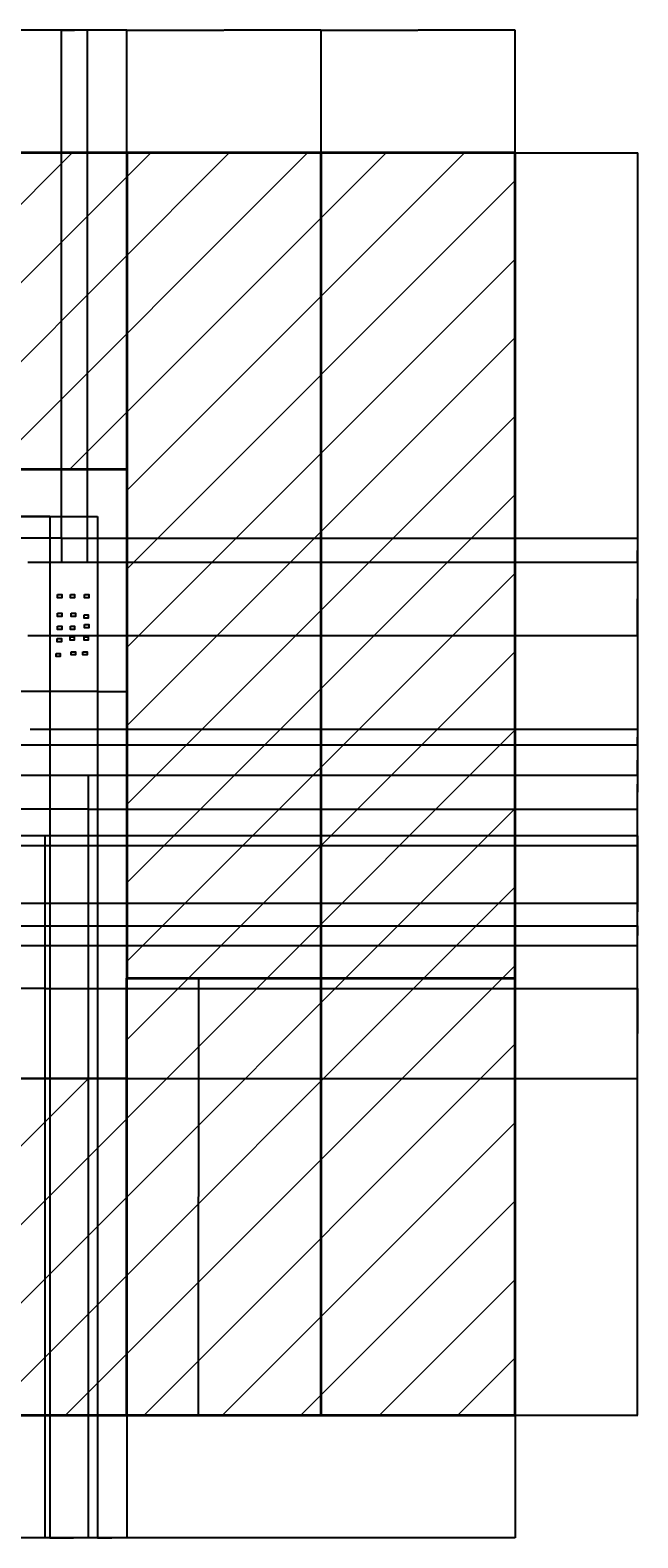
# Model space of a CAD drawing. Units: millimetres. Extents: x 2212 to 7718, y 1114 to 4219.
# Tile 5 of 5: x 6466 to 7718, y 1114 to 4219. Entities that reach past the tile are written whole.
import ezdxf

# ---------------------------------------------------------------- set-up
doc = ezdxf.new("R2010")
doc.units = ezdxf.units.MM
for name, color, linetype, lineweight in [('A-ANNO-DIMS', 2, 'Continuous', 18), ('A-ELEV-PATT', 8, 'Continuous', 13), ('A-EQPM', 4, 'Continuous', 25), ('A-FURN', 7, 'Continuous', 35)]:
    doc.layers.add(name, color=color, linetype=linetype, lineweight=lineweight)
doc.styles.get("Standard").update_dxf_attribs({"font": 'arial.ttf'})
doc.dimstyles.get("Standard").update_dxf_attribs({"dimtxt": 0.18, "dimasz": 0.18, "dimexe": 0.18, "dimexo": 0.0625, "dimgap": 0.09, "dimtad": 0, "dimtih": 1, "dimtoh": 1, "dimdec": 4, "dimzin": 0, "dimdsep": 46, "dimtxsty": 'Standard', "dimcen": 0.09, "dimadec": 0, "dimazin": 0, "dimtfac": 1, "dimtdec": 4, "dimtofl": 0, "dimtmove": 0, "dimatfit": 3, "dimfxl": 1, "dimtolj": 1, "dimtzin": 0, "dimarcsym": 0})

# ---------------------------------------------------------------- blocks, each defined once
blk = doc.blocks.new('*D7')
at = {"layer": 'A-ANNO-DIMS', "color": 0, "lineweight": -2, "transparency": 16777216}
for p, q in [((5865.1, 3966.2), (5865.1, 4218.9)), ((5865.3, 4218.7), (6264.9, 4218.7)), ((6665, 4218.7), (6265.4, 4218.7)), ((6665.1, 3966.2), (6665.1, 4218.9))]:
    blk.add_line(p, q, dxfattribs=at)
at = {"layer": 'A-ANNO-DIMS', "color": 0, "transparency": 16777216}
for points in [[(5865.3, 4218.7), (5865.3, 4218.7), (5865.1, 4218.7)], [(6665, 4218.7), (6665, 4218.7), (6665.1, 4218.7)]]:
    blk.add_solid(points, dxfattribs=at)
at = {"layer": 'Defpoints', "color": 0, "transparency": 16777216}
for p in [(6665.1, 4218.7), (5865.1, 3966.2), (6665.1, 3966.2)]:
    blk.add_point(p, dxfattribs=at)
at = {"layer": 'A-ANNO-DIMS', "color": 0, "transparency": 16777216, "insert": (6265.1, 4218.7), "char_height": 0.18, "attachment_point": 5}
blk.add_mtext('\\A1;800', dxfattribs=at)
blk = doc.blocks.new('*D8')
at = {"layer": 'A-ANNO-DIMS', "color": 0, "lineweight": -2, "transparency": 16777216}
for p, q in [((6665.1, 3966.2), (6665.1, 4218.9)), ((6665.3, 4218.7), (6864.8, 4218.7)), ((7065, 4218.7), (6865.4, 4218.7)), ((7065.1, 3966.2), (7065.1, 4218.9))]:
    blk.add_line(p, q, dxfattribs=at)
at = {"layer": 'A-ANNO-DIMS', "color": 0, "transparency": 16777216}
for points in [[(6665.3, 4218.7), (6665.3, 4218.7), (6665.1, 4218.7)], [(7065, 4218.7), (7065, 4218.7), (7065.1, 4218.7)]]:
    blk.add_solid(points, dxfattribs=at)
at = {"layer": 'Defpoints', "color": 0, "transparency": 16777216}
for p in [(7065.1, 4218.7), (6665.1, 3966.2), (7065.1, 3966.2)]:
    blk.add_point(p, dxfattribs=at)
at = {"layer": 'A-ANNO-DIMS', "color": 0, "transparency": 16777216, "insert": (6865.1, 4218.7), "char_height": 0.18, "attachment_point": 5}
blk.add_mtext('\\A1;400', dxfattribs=at)
blk = doc.blocks.new('*D9')
at = {"layer": 'A-ANNO-DIMS', "color": 0, "lineweight": -2, "transparency": 16777216}
for p, q in [((7065.1, 3966.2), (7065.1, 4218.9)), ((7065.3, 4218.7), (7264.8, 4218.7)), ((7465, 4218.7), (7265.4, 4218.7)), ((7465.1, 3966.2), (7465.1, 4218.9))]:
    blk.add_line(p, q, dxfattribs=at)
at = {"layer": 'A-ANNO-DIMS', "color": 0, "transparency": 16777216}
for points in [[(7065.3, 4218.7), (7065.3, 4218.7), (7065.1, 4218.7)], [(7465, 4218.7), (7465, 4218.7), (7465.1, 4218.7)]]:
    blk.add_solid(points, dxfattribs=at)
at = {"layer": 'Defpoints', "color": 0, "transparency": 16777216}
for p in [(7465.1, 4218.7), (7065.1, 3966.2), (7465.1, 3966.2)]:
    blk.add_point(p, dxfattribs=at)
at = {"layer": 'A-ANNO-DIMS', "color": 0, "transparency": 16777216, "insert": (7265.1, 4218.7), "char_height": 0.18, "attachment_point": 5}
blk.add_mtext('\\A1;400', dxfattribs=at)
blk = doc.blocks.new('*D18')
at = {"layer": 'A-ANNO-DIMS', "color": 0, "lineweight": -2, "transparency": 16777216}
for p, q in [((2465.1, 1366.1), (2465.1, 1113.5)), ((7465.1, 1366.1), (7465.1, 1113.5)), ((2465.3, 1113.7), (4964.8, 1113.7)), ((7465, 1113.7), (4965.5, 1113.7))]:
    blk.add_line(p, q, dxfattribs=at)
at = {"layer": 'A-ANNO-DIMS', "color": 0, "transparency": 16777216}
for points in [[(2465.3, 1113.7), (2465.3, 1113.7), (2465.1, 1113.7)], [(7465, 1113.7), (7465, 1113.7), (7465.1, 1113.7)]]:
    blk.add_solid(points, dxfattribs=at)
at = {"layer": 'Defpoints', "color": 0, "transparency": 16777216}
for p in [(2465.1, 1366.2), (7465.1, 1366.2), (7465.1, 1113.7)]:
    blk.add_point(p, dxfattribs=at)
at = {"layer": 'A-ANNO-DIMS', "color": 0, "transparency": 16777216, "insert": (4965.1, 1113.7), "char_height": 0.18, "attachment_point": 5}
blk.add_mtext('\\A1;5000', dxfattribs=at)
blk = doc.blocks.new('*D24')
at = {"layer": 'A-ANNO-DIMS', "color": 0, "lineweight": -2, "transparency": 16777216}
for p, q in [((7465.2, 3966.2), (7717.8, 3966.2)), ((7717.6, 3966), (7717.6, 2666.4)), ((7717.6, 1366.4), (7717.6, 2666)), ((7465.2, 1366.2), (7717.8, 1366.2))]:
    blk.add_line(p, q, dxfattribs=at)
at = {"layer": 'A-ANNO-DIMS', "color": 0, "transparency": 16777216}
for points in [[(7717.6, 3966), (7717.7, 3966), (7717.6, 3966.2)], [(7717.6, 1366.4), (7717.7, 1366.4), (7717.6, 1366.2)]]:
    blk.add_solid(points, dxfattribs=at)
at = {"layer": 'Defpoints', "color": 0, "transparency": 16777216}
for p in [(7465.1, 3966.2), (7717.6, 3966.2), (7465.1, 1366.2)]:
    blk.add_point(p, dxfattribs=at)
at = {"layer": 'A-ANNO-DIMS', "color": 0, "transparency": 16777216, "insert": (7717.6, 2666.2), "char_height": 0.18, "attachment_point": 5}
blk.add_mtext('\\A1;2600', dxfattribs=at)
blk = doc.blocks.new('*D25')
at = {"layer": 'A-ANNO-DIMS', "color": 0, "lineweight": -2, "transparency": 16777216}
for p, q in [((7065.1, 2266.4), (6812.5, 2266.4)), ((6812.6, 2266.2), (6812.6, 1816.5)), ((6812.6, 1366.4), (6812.6, 1816.1)), ((7065.1, 1366.2), (6812.5, 1366.2))]:
    blk.add_line(p, q, dxfattribs=at)
at = {"layer": 'A-ANNO-DIMS', "color": 0, "transparency": 16777216}
for points in [[(6812.6, 2266.2), (6812.7, 2266.2), (6812.6, 2266.4)], [(6812.6, 1366.4), (6812.7, 1366.4), (6812.6, 1366.2)]]:
    blk.add_solid(points, dxfattribs=at)
at = {"layer": 'Defpoints', "color": 0, "transparency": 16777216}
for p in [(6812.6, 2266.4), (7065.1, 2266.4), (7065.1, 1366.2)]:
    blk.add_point(p, dxfattribs=at)
at = {"layer": 'A-ANNO-DIMS', "color": 0, "transparency": 16777216, "insert": (6812.6, 1816.3), "char_height": 0.18, "attachment_point": 5}
blk.add_mtext('\\A1;900.2', dxfattribs=at)
blk = doc.blocks.new('*D26')
at = {"layer": 'A-ANNO-DIMS', "color": 0, "lineweight": -2, "transparency": 16777216}
for p, q in [((6665.1, 2059.6), (6412.5, 2059.6)), ((6412.6, 2059.4), (6412.6, 1713.1)), ((6412.6, 1366.4), (6412.6, 1712.7)), ((6665.1, 1366.2), (6412.5, 1366.2))]:
    blk.add_line(p, q, dxfattribs=at)
at = {"layer": 'A-ANNO-DIMS', "color": 0, "transparency": 16777216}
for points in [[(6412.6, 2059.4), (6412.7, 2059.4), (6412.6, 2059.6)], [(6412.6, 1366.4), (6412.7, 1366.4), (6412.6, 1366.2)]]:
    blk.add_solid(points, dxfattribs=at)
at = {"layer": 'Defpoints', "color": 0, "transparency": 16777216}
for p in [(6412.6, 2059.6), (6665.1, 2059.6), (6665.1, 1366.2)]:
    blk.add_point(p, dxfattribs=at)
at = {"layer": 'A-ANNO-DIMS', "color": 0, "transparency": 16777216, "insert": (6412.6, 1712.9), "char_height": 0.18, "attachment_point": 5}
blk.add_mtext('\\A1;693.4', dxfattribs=at)
blk = doc.blocks.new('*D36')
at = {"layer": 'A-ANNO-DIMS', "color": 0, "lineweight": -2, "transparency": 16777216}
for p, q in [((6460.9, 3122.9), (7717.8, 3122.9)), ((7717.6, 3122.7), (7717.6, 3047.7)), ((7717.6, 2972.4), (7717.6, 3047.3)), ((6460.9, 2972.2), (7717.8, 2972.2))]:
    blk.add_line(p, q, dxfattribs=at)
at = {"layer": 'A-ANNO-DIMS', "color": 0, "transparency": 16777216}
for points in [[(7717.6, 3122.7), (7717.7, 3122.7), (7717.6, 3122.9)], [(7717.6, 2972.4), (7717.7, 2972.4), (7717.6, 2972.2)]]:
    blk.add_solid(points, dxfattribs=at)
at = {"layer": 'Defpoints', "color": 0, "transparency": 16777216}
for p in [(6460.8, 3122.9), (7717.6, 3122.9), (6460.8, 2972.2)]:
    blk.add_point(p, dxfattribs=at)
at = {"layer": 'A-ANNO-DIMS', "color": 0, "transparency": 16777216, "insert": (7717.6, 3047.5), "char_height": 0.18, "attachment_point": 5}
blk.add_mtext('\\A1;150.68', dxfattribs=at)
blk = doc.blocks.new('*D38')
at = {"layer": 'A-ANNO-DIMS', "color": 0, "lineweight": -2, "transparency": 16777216}
for p, q in [((6506.1, 2856.7), (6506.1, 1113.5)), ((6604.3, 2856.7), (6604.3, 1113.5)), ((6506.2, 1113.7), (6554.8, 1113.7)), ((6604.1, 1113.7), (6555.6, 1113.7))]:
    blk.add_line(p, q, dxfattribs=at)
at = {"layer": 'A-ANNO-DIMS', "color": 0, "transparency": 16777216}
for points in [[(6506.2, 1113.7), (6506.2, 1113.7), (6506.1, 1113.7)], [(6604.1, 1113.7), (6604.1, 1113.7), (6604.3, 1113.7)]]:
    blk.add_solid(points, dxfattribs=at)
at = {"layer": 'Defpoints', "color": 0, "transparency": 16777216}
for p in [(6506.1, 2856.7), (6604.3, 2856.7), (6604.3, 1113.7)]:
    blk.add_point(p, dxfattribs=at)
at = {"layer": 'A-ANNO-DIMS', "color": 0, "transparency": 16777216, "insert": (6555.2, 1113.7), "char_height": 0.18, "attachment_point": 5}
blk.add_mtext('\\A1;98.24', dxfattribs=at)
blk = doc.blocks.new('*D39')
at = {"layer": 'A-ANNO-DIMS', "color": 0, "lineweight": -2, "transparency": 16777216}
for p, q in [((6604.3, 2856.7), (6604.3, 1113.5)), ((6665.1, 2856.7), (6665.1, 1113.5)), ((6604.5, 1113.7), (6634.3, 1113.7)), ((6665, 1113.7), (6635.1, 1113.7))]:
    blk.add_line(p, q, dxfattribs=at)
at = {"layer": 'A-ANNO-DIMS', "color": 0, "transparency": 16777216}
for points in [[(6604.5, 1113.7), (6604.5, 1113.7), (6604.3, 1113.7)], [(6665, 1113.7), (6665, 1113.7), (6665.1, 1113.7)]]:
    blk.add_solid(points, dxfattribs=at)
at = {"layer": 'Defpoints', "color": 0, "transparency": 16777216}
for p in [(6604.3, 2856.7), (6665.1, 2856.7), (6665.1, 1113.7)]:
    blk.add_point(p, dxfattribs=at)
at = {"layer": 'A-ANNO-DIMS', "color": 0, "transparency": 16777216, "insert": (6634.7, 1113.7), "char_height": 0.18, "attachment_point": 5}
blk.add_mtext('\\A1;60.83', dxfattribs=at)
blk = doc.blocks.new('*D40')
at = {"layer": 'A-ANNO-DIMS', "color": 0, "lineweight": -2, "transparency": 16777216}
for p, q in [((6530.5, 3172.4), (6530.5, 4218.9)), ((6530.6, 4218.7), (6556.8, 4218.7)), ((6583.8, 4218.7), (6557.6, 4218.7)), ((6584, 3172.4), (6584, 4218.9))]:
    blk.add_line(p, q, dxfattribs=at)
at = {"layer": 'A-ANNO-DIMS', "color": 0, "transparency": 16777216}
for points in [[(6530.6, 4218.7), (6530.6, 4218.7), (6530.5, 4218.7)], [(6583.8, 4218.7), (6583.8, 4218.7), (6584, 4218.7)]]:
    blk.add_solid(points, dxfattribs=at)
at = {"layer": 'Defpoints', "color": 0, "transparency": 16777216}
for p in [(6584, 4218.7), (6530.5, 3172.4), (6584, 3172.4)]:
    blk.add_point(p, dxfattribs=at)
at = {"layer": 'A-ANNO-DIMS', "color": 0, "transparency": 16777216, "insert": (6557.2, 4218.7), "char_height": 0.18, "attachment_point": 5}
blk.add_mtext('\\A1;53.54', dxfattribs=at)
blk = doc.blocks.new('*D41')
at = {"layer": 'A-ANNO-DIMS', "color": 0, "lineweight": -2, "transparency": 16777216}
for p, q in [((6584.1, 3172.4), (7717.8, 3172.4)), ((7717.6, 3172.2), (7717.6, 3147.8)), ((7717.6, 3123), (7717.6, 3147.4)), ((6584.1, 3122.9), (7717.8, 3122.9))]:
    blk.add_line(p, q, dxfattribs=at)
at = {"layer": 'A-ANNO-DIMS', "color": 0, "transparency": 16777216}
for points in [[(7717.6, 3172.2), (7717.7, 3172.2), (7717.6, 3172.4)], [(7717.6, 3123), (7717.7, 3123), (7717.6, 3122.9)]]:
    blk.add_solid(points, dxfattribs=at)
at = {"layer": 'Defpoints', "color": 0, "transparency": 16777216}
for p in [(6584, 3172.4), (7717.6, 3172.4), (6584, 3122.9)]:
    blk.add_point(p, dxfattribs=at)
at = {"layer": 'A-ANNO-DIMS', "color": 0, "transparency": 16777216, "insert": (7717.6, 3147.6), "char_height": 0.18, "attachment_point": 5}
blk.add_mtext('\\A1;49.51', dxfattribs=at)
blk = doc.blocks.new('*D42')
at = {"layer": 'A-ANNO-DIMS', "color": 0, "lineweight": -2, "transparency": 16777216}
for p, q in [((6506, 3217.2), (2212.5, 3217.2)), ((2212.6, 3217.1), (2212.6, 3195)), ((6530.4, 3172.4), (2212.5, 3172.4)), ((2212.6, 3172.6), (2212.6, 3194.6))]:
    blk.add_line(p, q, dxfattribs=at)
at = {"layer": 'A-ANNO-DIMS', "color": 0, "transparency": 16777216}
for points in [[(2212.6, 3217.1), (2212.7, 3217.1), (2212.6, 3217.2)], [(2212.6, 3172.6), (2212.7, 3172.6), (2212.6, 3172.4)]]:
    blk.add_solid(points, dxfattribs=at)
at = {"layer": 'Defpoints', "color": 0, "transparency": 16777216}
for p in [(6506.1, 3217.2), (2212.6, 3172.4), (6530.5, 3172.4)]:
    blk.add_point(p, dxfattribs=at)
at = {"layer": 'A-ANNO-DIMS', "color": 0, "transparency": 16777216, "insert": (2212.6, 3194.8), "char_height": 0.18, "attachment_point": 5}
blk.add_mtext('\\A1;44.855', dxfattribs=at)
blk = doc.blocks.new('*D47')
at = {"layer": 'A-ANNO-DIMS', "color": 0, "lineweight": -2, "transparency": 16777216}
for p, q in [((6465.8, 2779.3), (7717.8, 2779.3)), ((7717.6, 2779.1), (7717.6, 2763.2)), ((6665.2, 2746.8), (7717.8, 2746.8)), ((7717.6, 2747), (7717.6, 2762.9))]:
    blk.add_line(p, q, dxfattribs=at)
at = {"layer": 'A-ANNO-DIMS', "color": 0, "transparency": 16777216}
for points in [[(7717.6, 2779.1), (7717.7, 2779.1), (7717.6, 2779.3)], [(7717.6, 2747), (7717.7, 2747), (7717.6, 2746.8)]]:
    blk.add_solid(points, dxfattribs=at)
at = {"layer": 'Defpoints', "color": 0, "transparency": 16777216}
for p in [(6465.7, 2779.3), (6665.1, 2746.8), (7717.6, 2746.8)]:
    blk.add_point(p, dxfattribs=at)
at = {"layer": 'A-ANNO-DIMS', "color": 0, "transparency": 16777216, "insert": (7717.6, 2763), "char_height": 0.18, "attachment_point": 5}
blk.add_mtext('\\A1;32.5', dxfattribs=at)
blk = doc.blocks.new('*D48')
at = {"layer": 'A-ANNO-DIMS', "color": 0, "lineweight": -2, "transparency": 16777216}
for p, q in [((5929, 2614.5), (5929, 1113.5)), ((6585.5, 2614.5), (6585.5, 1113.5)), ((5929.2, 1113.7), (6256.9, 1113.7)), ((6585.3, 1113.7), (6257.7, 1113.7))]:
    blk.add_line(p, q, dxfattribs=at)
at = {"layer": 'A-ANNO-DIMS', "color": 0, "transparency": 16777216}
for points in [[(5929.2, 1113.7), (5929.2, 1113.7), (5929, 1113.7)], [(6585.3, 1113.7), (6585.3, 1113.7), (6585.5, 1113.7)]]:
    blk.add_solid(points, dxfattribs=at)
at = {"layer": 'Defpoints', "color": 0, "transparency": 16777216}
for p in [(5929, 2614.6), (6585.5, 2614.6), (6585.5, 1113.7)]:
    blk.add_point(p, dxfattribs=at)
at = {"layer": 'A-ANNO-DIMS', "color": 0, "transparency": 16777216, "insert": (6257.3, 1113.7), "char_height": 0.18, "attachment_point": 5}
blk.add_mtext('\\A1;656.5', dxfattribs=at)
blk = doc.blocks.new('*D49')
at = {"layer": 'A-ANNO-DIMS', "color": 0, "lineweight": -2, "transparency": 16777216}
for p, q in [((6585.6, 2684.5), (7717.8, 2684.5)), ((7717.6, 2684.4), (7717.6, 2649.7)), ((7717.6, 2614.7), (7717.6, 2649.4)), ((6585.6, 2614.6), (7717.8, 2614.6))]:
    blk.add_line(p, q, dxfattribs=at)
at = {"layer": 'A-ANNO-DIMS', "color": 0, "transparency": 16777216}
for points in [[(7717.6, 2684.4), (7717.7, 2684.4), (7717.6, 2684.5)], [(7717.6, 2614.7), (7717.7, 2614.7), (7717.6, 2614.6)]]:
    blk.add_solid(points, dxfattribs=at)
at = {"layer": 'Defpoints', "color": 0, "transparency": 16777216}
for p in [(6585.5, 2684.5), (7717.6, 2684.5), (6585.5, 2614.6)]:
    blk.add_point(p, dxfattribs=at)
at = {"layer": 'A-ANNO-DIMS', "color": 0, "transparency": 16777216, "insert": (7717.6, 2649.5), "char_height": 0.18, "attachment_point": 5}
blk.add_mtext('\\A1;69.96', dxfattribs=at)
blk = doc.blocks.new('*D51')
at = {"layer": 'A-ANNO-DIMS', "color": 0, "lineweight": -2, "transparency": 16777216}
for p, q in [((6665.2, 2746.8), (7717.8, 2746.8)), ((7717.6, 2746.6), (7717.6, 2715.8)), ((7717.6, 2684.7), (7717.6, 2715.5)), ((6585.6, 2684.5), (7717.8, 2684.5))]:
    blk.add_line(p, q, dxfattribs=at)
at = {"layer": 'A-ANNO-DIMS', "color": 0, "transparency": 16777216}
for points in [[(7717.6, 2746.6), (7717.7, 2746.6), (7717.6, 2746.8)], [(7717.6, 2684.7), (7717.7, 2684.7), (7717.6, 2684.5)]]:
    blk.add_solid(points, dxfattribs=at)
at = {"layer": 'Defpoints', "color": 0, "transparency": 16777216}
for p in [(6665.1, 2746.8), (7717.6, 2746.8), (6585.5, 2684.5)]:
    blk.add_point(p, dxfattribs=at)
at = {"layer": 'A-ANNO-DIMS', "color": 0, "transparency": 16777216, "insert": (7717.6, 2715.7), "char_height": 0.18, "attachment_point": 5}
blk.add_mtext('\\A1;62.26', dxfattribs=at)
blk = doc.blocks.new('*D52')
at = {"layer": 'A-ANNO-DIMS', "color": 0, "lineweight": -2, "transparency": 16777216}
for p, q in [((5994.7, 2245), (5994.7, 1113.5)), ((6495.8, 2245), (6495.8, 1113.5)), ((5994.9, 1113.7), (6244.9, 1113.7)), ((6495.6, 1113.7), (6245.6, 1113.7))]:
    blk.add_line(p, q, dxfattribs=at)
at = {"layer": 'A-ANNO-DIMS', "color": 0, "transparency": 16777216}
for points in [[(5994.9, 1113.7), (5994.9, 1113.7), (5994.7, 1113.7)], [(6495.6, 1113.7), (6495.6, 1113.7), (6495.8, 1113.7)]]:
    blk.add_solid(points, dxfattribs=at)
at = {"layer": 'Defpoints', "color": 0, "transparency": 16777216}
for p in [(5994.7, 2245.1), (6495.8, 2245.1), (6495.8, 1113.7)]:
    blk.add_point(p, dxfattribs=at)
at = {"layer": 'A-ANNO-DIMS', "color": 0, "transparency": 16777216, "insert": (6245.3, 1113.7), "char_height": 0.18, "attachment_point": 5}
blk.add_mtext('\\A1;501.1', dxfattribs=at)
blk = doc.blocks.new('*D53')
at = {"layer": 'A-ANNO-DIMS', "color": 0, "lineweight": -2, "transparency": 16777216}
for p, q in [((6495.9, 2559.9), (7717.8, 2559.9)), ((7717.6, 2559.7), (7717.6, 2402.7)), ((7717.6, 2245.3), (7717.6, 2402.3)), ((6495.9, 2245.1), (7717.8, 2245.1))]:
    blk.add_line(p, q, dxfattribs=at)
at = {"layer": 'A-ANNO-DIMS', "color": 0, "transparency": 16777216}
for points in [[(7717.6, 2559.7), (7717.7, 2559.7), (7717.6, 2559.9)], [(7717.6, 2245.3), (7717.7, 2245.3), (7717.6, 2245.1)]]:
    blk.add_solid(points, dxfattribs=at)
at = {"layer": 'Defpoints', "color": 0, "transparency": 16777216}
for p in [(6495.8, 2559.9), (7717.6, 2559.9), (6495.8, 2245.1)]:
    blk.add_point(p, dxfattribs=at)
at = {"layer": 'A-ANNO-DIMS', "color": 0, "transparency": 16777216, "insert": (7717.6, 2402.5), "char_height": 0.18, "attachment_point": 5}
blk.add_mtext('\\A1;314.84', dxfattribs=at)
blk = doc.blocks.new('*D55')
at = {"layer": 'A-ANNO-DIMS', "color": 0, "lineweight": -2, "transparency": 16777216}
for p, q in [((6495.9, 2245.1), (7717.8, 2245.1)), ((7717.6, 2244.9), (7717.6, 2152.5)), ((7717.6, 2059.8), (7717.6, 2152.2)), ((6665.2, 2059.6), (7717.8, 2059.6))]:
    blk.add_line(p, q, dxfattribs=at)
at = {"layer": 'A-ANNO-DIMS', "color": 0, "transparency": 16777216}
for points in [[(7717.6, 2244.9), (7717.7, 2244.9), (7717.6, 2245.1)], [(7717.6, 2059.8), (7717.7, 2059.8), (7717.6, 2059.6)]]:
    blk.add_solid(points, dxfattribs=at)
at = {"layer": 'Defpoints', "color": 0, "transparency": 16777216}
for p in [(6495.8, 2245.1), (6665.1, 2059.6), (7717.6, 2059.6)]:
    blk.add_point(p, dxfattribs=at)
at = {"layer": 'A-ANNO-DIMS', "color": 0, "transparency": 16777216, "insert": (7717.6, 2152.3), "char_height": 0.18, "attachment_point": 5}
blk.add_mtext('\\A1;185.46', dxfattribs=at)
blk = doc.blocks.new('*D71')
at = {"layer": 'A-ANNO-DIMS', "color": 0, "lineweight": -2, "transparency": 16777216}
for p, q in [((5608.2, 2374.1), (7717.8, 2374.1)), ((7717.6, 2373.9), (7717.6, 2353.9)), ((5537.5, 2333.4), (7717.8, 2333.4)), ((7717.6, 2333.5), (7717.6, 2353.5))]:
    blk.add_line(p, q, dxfattribs=at)
at = {"layer": 'A-ANNO-DIMS', "color": 0, "transparency": 16777216}
for points in [[(7717.6, 2373.9), (7717.7, 2373.9), (7717.6, 2374.1)], [(7717.6, 2333.5), (7717.7, 2333.5), (7717.6, 2333.4)]]:
    blk.add_solid(points, dxfattribs=at)
at = {"layer": 'Defpoints', "color": 0, "transparency": 16777216}
for p in [(5608.2, 2374.1), (7717.6, 2374.1), (5537.5, 2333.4)]:
    blk.add_point(p, dxfattribs=at)
at = {"layer": 'A-ANNO-DIMS', "color": 0, "transparency": 16777216, "insert": (7717.6, 2353.7), "char_height": 0.18, "attachment_point": 5}
blk.add_mtext('\\A1;40.726', dxfattribs=at)
blk = doc.blocks.new('*D73')
at = {"layer": 'A-ANNO-DIMS', "color": 0, "lineweight": -2, "transparency": 16777216}
for p, q in [((5284.8, 2539.3), (7717.8, 2539.3)), ((7717.6, 2539.1), (7717.6, 2480.2)), ((7717.6, 2420.9), (7717.6, 2479.8)), ((5329.4, 2420.7), (7717.8, 2420.7))]:
    blk.add_line(p, q, dxfattribs=at)
at = {"layer": 'A-ANNO-DIMS', "color": 0, "transparency": 16777216}
for points in [[(7717.6, 2539.1), (7717.7, 2539.1), (7717.6, 2539.3)], [(7717.6, 2420.9), (7717.7, 2420.9), (7717.6, 2420.7)]]:
    blk.add_solid(points, dxfattribs=at)
at = {"layer": 'Defpoints', "color": 0, "transparency": 16777216}
for p in [(5284.8, 2539.3), (7717.6, 2539.3), (5329.3, 2420.7)]:
    blk.add_point(p, dxfattribs=at)
at = {"layer": 'A-ANNO-DIMS', "color": 0, "transparency": 16777216, "insert": (7717.6, 2480), "char_height": 0.18, "attachment_point": 5}
blk.add_mtext('\\A1;118.60', dxfattribs=at)

msp = doc.modelspace()

# ---------------------------------------------------------------- hatches: boundary and pattern name
at = {"layer": 'A-ELEV-PATT'}
h = msp.add_hatch(dxfattribs=at)
h.set_pattern_fill('ANSI31', color=256, scale=36)
h.paths.add_polyline_path([(3153.454, 3966.1829), (2465.1412, 3966.1829), (2465.1412, 3121.3339), (3153.454, 3121.3339)])
h.paths.add_polyline_path([(3659.2976, 3966.1829), (3153.454, 3966.1829), (3153.454, 3121.3339), (3659.2976, 3121.3339)])
h.paths.add_polyline_path([(4165.1412, 3966.1829), (3659.2976, 3966.1829), (3659.2976, 3121.3339), (4165.1412, 3121.3339)])
h.paths.add_polyline_path([(3365.1412, 2266.3983), (2465.1412, 2266.3983), (2465.1412, 1366.1829), (3365.1412, 1366.1829)])
h.paths.add_polyline_path([(4165.1412, 2266.3983), (3365.1412, 2266.3983), (3365.1412, 1366.1829), (4165.1412, 1366.1829)])
h.paths.add_polyline_path([(4965.1412, 2266.3983), (4165.1412, 2266.3983), (4165.1412, 1366.1829), (4965.1412, 1366.1829)])
h.paths.add_polyline_path([(5765.1412, 2266.3983), (4965.1412, 2266.3983), (4965.1412, 1366.1829), (5765.1412, 1366.1829)])
h.paths.add_polyline_path([(6665.1412, 2059.6125), (5865.1412, 2059.6125), (5865.1412, 1366.1829), (6665.1412, 1366.1829)])
h.paths.add_polyline_path([(7465.1412, 2266.3983), (7065.1412, 2266.3983), (7065.1412, 1366.1829), (7465.1412, 1366.1829)])
h.paths.add_polyline_path([(7065.1412, 2266.3983), (6665.1412, 2266.3983), (6665.1412, 1366.1829), (7065.1412, 1366.1829)])
h.paths.add_polyline_path([(7465.1412, 3966.1829), (7065.1412, 3966.1829), (7065.1412, 2266.3983), (7465.1412, 2266.3983)])
h.paths.add_polyline_path([(7065.1412, 3966.1829), (6665.1412, 3966.1829), (6665.1412, 2266.3983), (7065.1412, 2266.3983)])
h.paths.add_polyline_path([(6665.1412, 3966.1829), (6027.7806, 3966.1829), (6027.7806, 3314.3715), (6665.1412, 3314.3715)])
h.paths.add_polyline_path([(5245.7331, 3966.1829), (4821.5849, 3966.1829), (4821.5849, 3216.3983), (4356.7186, 3216.3983), (4356.7186, 3121.3339), (5503.6152, 3121.3339), (5720.779, 3121.3339), (5720.779, 3216.3983), (5245.7331, 3216.3983)])

# ---------------------------------------------------------------- linework, layer by layer
at = {"layer": 'A-EQPM'}
for p, q in [((5865.1412, 3217.2303), (6604.3074, 3217.2303)), ((6506.0666, 3217.2303), (6506.0666, 2856.7409)), ((6604.3074, 3217.2303), (6604.3074, 2856.7409)), ((6530.4592, 3172.3755), (6583.9972, 3172.3755)), ((6530.4592, 3172.3755), (6530.4592, 3122.866)), ((6583.9972, 3122.866), (6583.9972, 3172.3755)), ((6530.4592, 3122.866), (6583.9972, 3122.866)), ((6530.4592, 3122.866), (6583.9972, 3122.866)), ((6604.3074, 2856.7409), (5865.1412, 2856.7409)), ((6604.3074, 2856.7409), (6665.1412, 2856.7409)), ((5865.1412, 2746.7954), (6665.1412, 2746.7954)), ((5865.1412, 2059.6125), (6665.1412, 2059.6125))]:
    msp.add_line(p, q, dxfattribs=at)
for points in [[(6522.4501, 3056.2527), (6530.9747, 3056.2527), (6530.9747, 3049.4388), (6522.4501, 3049.4388)], [(6548.8763, 3056.2527), (6557.401, 3056.2527), (6557.401, 3049.4388), (6548.8763, 3049.4388)], [(6577.86, 3056.2527), (6586.3846, 3056.2527), (6586.3846, 3049.4388), (6577.86, 3049.4388)], [(6522.4501, 3017.9249), (6530.9747, 3017.9249), (6530.9747, 3011.1111), (6522.4501, 3011.1111)], [(6550.5813, 3017.9249), (6559.1059, 3017.9249), (6559.1059, 3011.1111), (6550.5813, 3011.1111)], [(6577.0075, 3014.518), (6585.5321, 3014.518), (6585.5321, 3007.7042), (6577.0075, 3007.7042)], [(6522.4501, 2991.5213), (6530.9747, 2991.5213), (6530.9747, 2984.7075), (6522.4501, 2984.7075)], [(6548.8763, 2991.5213), (6557.401, 2991.5213), (6557.401, 2984.7075), (6548.8763, 2984.7075)], [(6577.86, 2994.9283), (6586.3846, 2994.9283), (6586.3846, 2988.1144), (6577.86, 2988.1144)], [(6521.5976, 2965.9695), (6530.1222, 2965.9695), (6530.1222, 2959.1557), (6521.5976, 2959.1557)], [(6548.0239, 2969.3764), (6556.5485, 2969.3764), (6556.5485, 2962.5626), (6548.0239, 2962.5626)], [(6577.0075, 2969.3764), (6585.5321, 2969.3764), (6585.5321, 2962.5626), (6577.0075, 2962.5626)], [(6519.0402, 2935.3073), (6527.5648, 2935.3073), (6527.5648, 2928.4935), (6519.0402, 2928.4935)], [(6550.5813, 2938.7142), (6559.1059, 2938.7142), (6559.1059, 2931.9004), (6550.5813, 2931.9004)], [(6574.4502, 2938.7142), (6582.9748, 2938.7142), (6582.9748, 2931.9004), (6574.4502, 2931.9004)], [(5929.0495, 2684.5306), (6585.5248, 2684.5306), (6585.5248, 2614.5667), (5929.0495, 2614.5667)], [(5994.697, 2559.9075), (6495.8065, 2559.9075), (6495.8065, 2245.0701), (5994.697, 2245.0701)]]:
    msp.add_lwpolyline(points, close=True, dxfattribs=at)
at = {"layer": 'A-FURN'}
for p, q in [((7465.1412, 3966.1829), (5865.1412, 3966.1829)), ((6665.1412, 3966.1829), (6665.1412, 2266.3983)), ((7065.1412, 2266.3983), (7065.1412, 3966.1829)), ((7465.1412, 2266.3983), (7465.1412, 3966.1829)), ((5865.1412, 3314.3715), (6665.1412, 3314.3715)), ((6665.1412, 1366.1829), (6665.1412, 2266.3983)), ((6665.1412, 2266.3983), (7465.1412, 2266.3983)), ((7065.1412, 1366.1829), (7065.1412, 2266.3983)), ((7465.1412, 1366.1829), (7465.1412, 2266.3983)), ((5865.1412, 1366.1829), (6665.1412, 1366.1829)), ((6665.1412, 1366.1829), (7465.1412, 1366.1829))]:
    msp.add_line(p, q, dxfattribs=at)

# ---------------------------------------------------------------- dimensions: what is measured, and where the dimension line sits
at = {"layer": 'A-ANNO-DIMS'}
for base, p1, p2, override, picture, middle in [((6665.1412, 4218.6829), (5865.1412, 3966.1829), (6665.1412, 3966.1829), {"dimdec": 0, "dimlfac": 1, "dimrnd": 0, "dimzin": 0, "dimdsep": 46, "dimlunit": 2}, '*D7', (6265.1412, 4218.6829)), ((6583.9972, 4218.6829), (6530.4592, 3172.3755), (6583.9972, 3172.3755), {"dimdec": 2, "dimlfac": 1, "dimrnd": 0, "dimzin": 0, "dimdsep": 46, "dimlunit": 2}, '*D40', (6557.2282, 4218.6829)), ((7065.1412, 4218.6829), (6665.1412, 3966.1829), (7065.1412, 3966.1829), {"dimdec": 0, "dimlfac": 1, "dimrnd": 0, "dimzin": 0, "dimdsep": 46, "dimlunit": 2}, '*D8', (6865.1412, 4218.6829)), ((7465.1412, 4218.6829), (7065.1412, 3966.1829), (7465.1412, 3966.1829), {"dimdec": 0, "dimlfac": 1, "dimrnd": 0, "dimzin": 0, "dimdsep": 46, "dimlunit": 2}, '*D9', (7265.1412, 4218.6829)), ((6604.3074, 1113.6829), (6506.0666, 2856.7409), (6604.3074, 2856.7409), {"dimdec": 2, "dimlfac": 1, "dimrnd": 0, "dimzin": 0, "dimdsep": 46, "dimlunit": 2}, '*D38', (6555.187, 1113.6829)), ((6665.1412, 1113.6829), (6604.3074, 2856.7409), (6665.1412, 2856.7409), {"dimdec": 2, "dimlfac": 1, "dimrnd": 0, "dimzin": 0, "dimdsep": 46, "dimlunit": 2}, '*D39', (6634.7243, 1113.6829)), ((6585.5248, 1113.6829), (5929.0495, 2614.5667), (6585.5248, 2614.5667), {"dimdec": 1, "dimlfac": 1, "dimrnd": 0, "dimzin": 0, "dimdsep": 46, "dimlunit": 2}, '*D48', (6257.2872, 1113.6829)), ((6495.8065, 1113.6829), (5994.697, 2245.0701), (6495.8065, 2245.0701), {"dimdec": 1, "dimlfac": 1, "dimrnd": 0, "dimzin": 0, "dimdsep": 46, "dimlunit": 2}, '*D52', (6245.2518, 1113.6829)), ((7465.1412, 1113.6829), (2465.1412, 1366.1829), (7465.1412, 1366.1829), {"dimdec": 0, "dimlfac": 1, "dimrnd": 0, "dimzin": 0, "dimdsep": 46, "dimlunit": 2}, '*D18', (4965.1412, 1113.6829))]:
    dim = msp.add_linear_dim(base=base, p1=p1, p2=p2, dimstyle='Standard', override=override, dxfattribs=at)
    dim.commit()
    dim.dimension.update_dxf_attribs({"geometry": picture, "text_midpoint": middle})
for base, p1, p2, override, picture, middle in [((7717.6412, 3966.1829), (7465.1412, 1366.1829), (7465.1412, 3966.1829), {"dimdec": 0, "dimlfac": 1, "dimrnd": 0, "dimzin": 0, "dimdsep": 46, "dimlunit": 2}, '*D24', (7717.6412, 2666.1829)), ((2212.6412, 3172.3755), (6506.0666, 3217.2303), (6530.4592, 3172.3755), {"dimdec": 3, "dimlfac": 1, "dimrnd": 0, "dimzin": 0, "dimdsep": 46, "dimlunit": 2}, '*D42', (2212.6412, 3194.8029)), ((7717.6412, 3172.3755), (6583.9972, 3122.866), (6583.9972, 3172.3755), {"dimdec": 2, "dimlfac": 1, "dimrnd": 0, "dimzin": 0, "dimdsep": 46, "dimlunit": 2}, '*D41', (7717.6412, 3147.6207)), ((7717.6412, 3122.866), (6460.8234, 2972.1846), (6460.8234, 3122.866), {"dimdec": 2, "dimlfac": 1, "dimrnd": 0, "dimzin": 0, "dimdsep": 46, "dimlunit": 2}, '*D36', (7717.6412, 3047.5253)), ((7717.6412, 2746.7954), (6465.7339, 2779.2966), (6665.1412, 2746.7954), {"dimdec": 1, "dimlfac": 1, "dimrnd": 0, "dimzin": 0, "dimdsep": 46, "dimlunit": 2}, '*D47', (7717.6412, 2763.046)), ((7717.6412, 2746.7954), (6585.5248, 2684.5306), (6665.1412, 2746.7954), {"dimdec": 2, "dimlfac": 1, "dimrnd": 0, "dimzin": 0, "dimdsep": 46, "dimlunit": 2}, '*D51', (7717.6412, 2715.663)), ((7717.6412, 2684.5306), (6585.5248, 2614.5667), (6585.5248, 2684.5306), {"dimdec": 2, "dimlfac": 1, "dimrnd": 0, "dimzin": 0, "dimdsep": 46, "dimlunit": 2}, '*D49', (7717.6412, 2649.5487)), ((7717.6412, 2559.9075), (6495.8065, 2245.0701), (6495.8065, 2559.9075), {"dimdec": 2, "dimlfac": 1, "dimrnd": 0, "dimzin": 0, "dimdsep": 46, "dimlunit": 2}, '*D53', (7717.6412, 2402.4888)), ((7717.6412, 2539.2808), (5329.3388, 2420.6771), (5284.7847, 2539.2808), {"dimdec": 2, "dimlfac": 1, "dimrnd": 0, "dimzin": 0, "dimdsep": 46, "dimlunit": 2}, '*D73', (7717.6412, 2479.979)), ((7717.64116, 2374.09375), (5537.48322, 2333.36822), (5608.17143, 2374.09375), {"dimdec": 3, "dimlfac": 1, "dimrnd": 0, "dimzin": 0, "dimdsep": 46, "dimlunit": 2}, '*D71', (7717.64116, 2353.73098)), ((7717.6412, 2059.6125), (6495.8065, 2245.0701), (6665.1412, 2059.6125), {"dimdec": 2, "dimlfac": 1, "dimrnd": 0, "dimzin": 0, "dimdsep": 46, "dimlunit": 2}, '*D55', (7717.6412, 2152.3413)), ((6812.6412, 2266.3983), (7065.1412, 1366.1829), (7065.1412, 2266.3983), {"dimdec": 1, "dimlfac": 1, "dimrnd": 0, "dimzin": 0, "dimdsep": 46, "dimlunit": 2}, '*D25', (6812.6412, 1816.2906)), ((6412.6412, 2059.6125), (6665.1412, 1366.1829), (6665.1412, 2059.6125), {"dimdec": 1, "dimlfac": 1, "dimrnd": 0, "dimzin": 0, "dimdsep": 46, "dimlunit": 2}, '*D26', (6412.6412, 1712.8977))]:
    dim = msp.add_linear_dim(base=base, p1=p1, p2=p2, angle=90, dimstyle='Standard', override=override, dxfattribs=at)
    dim.commit()
    dim.dimension.update_dxf_attribs({"geometry": picture, "text_midpoint": middle})

doc.saveas('drawing.dxf')
